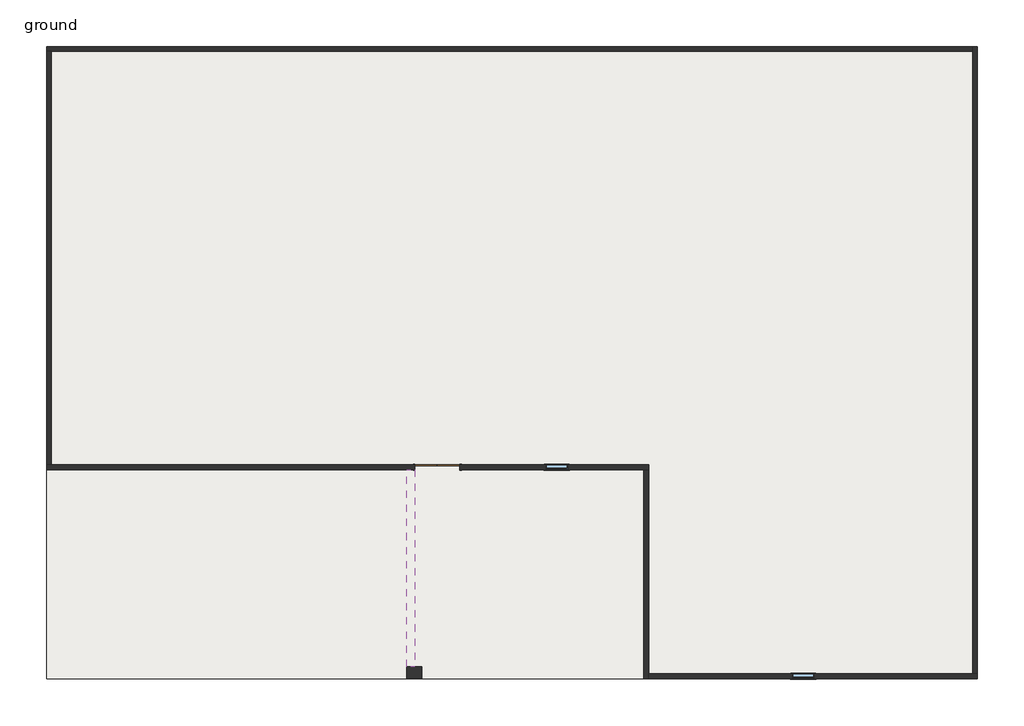
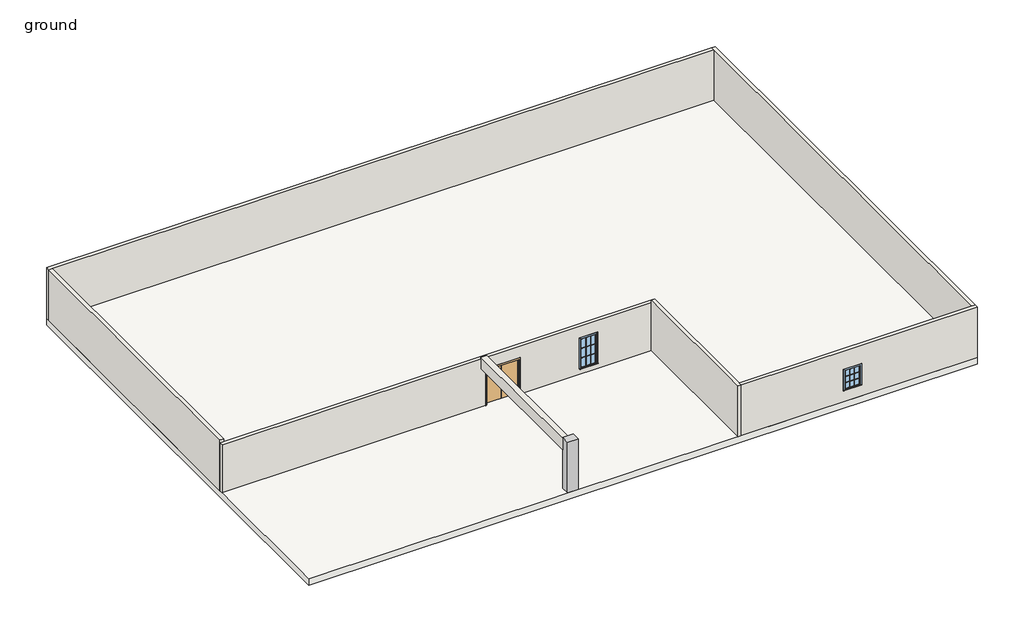
# One storey: 7 walls, 2 windows, 1 column, 1 door, 1 slab.
"""IFC4 building model written with IfcOpenShell, lengths in millimetres."""

from ifc_helpers import new_model, si_unit, frame, origin, place, context, project, spatial, polyline, outline, extrude, faceted_brep, transform, mapped, element, save
from components import m_rectangular_column_475_x_610mm_5ff218ee, door_db0c0681, walls_2_walls_2_334e7359, window_ddc5d35f, window_0c844ac8

model = new_model("IFC4")

# Units and contexts
model_context = context("Model", 3, world=origin())
ifc_project = project(units=[si_unit("LENGTHUNIT", "METRE", prefix="MILLI")], contexts=[model_context])

# Site, building, storey
site = spatial("IfcSite", under=ifc_project)
building = spatial("IfcBuilding", under=site)
storey = spatial("IfcBuildingStorey", under=building, Name="ground", Elevation=0.0)

# Column
placement = place(None, origin())
m_rectangular_column_475_x_610mm_shape = m_rectangular_column_475_x_610mm_5ff218ee(model_context)
element("IfcColumn", 1, ObjectType="M_Rectangular Column : 475 x 610mm", at=placement, inside=storey, context=model_context, shape_type="MappedRepresentation", body=[
    mapped(m_rectangular_column_475_x_610mm_shape, transform((-2824.5479903, -9080.6874979, 0.0), x_axis=(1.0, 0.0, 0.0), y_axis=(0.0, 1.0, 0.0), z_axis=(0.0, 0.0, 1.0))),
])

# Door
door_shape = door_db0c0681(model_context)
element("IfcDoor", 2, ObjectType="Door-Double-Flush_Panel : 72\" x 84\"", at=placement, inside=storey, context=model_context, shape_type="MappedRepresentation", body=[
    mapped(door_shape, transform((-1883.9625081, -698.6874979, 0.0), x_axis=(1.0, 0.0, 0.0), y_axis=(0.0, 1.0, 0.0), z_axis=(0.0, 0.0, 1.0))),
])

# Slab
element("IfcSlab", 3, ObjectType="Generic Floor - 400mm", at=placement, inside=storey, context=model_context, shape_type="SweptSolid", body=[
    extrude(outline(polyline([(20161.6374919, 16470.1125021), (20161.6374919, -9333.0874979), (-17833.5625081, -9333.0874979), (-17833.5625081, 16470.1125021), (20161.6374919, 16470.1125021)])), frame((0.0, 0.0, -400.0), z_axis=(0.0, 0.0, 1.0), x_axis=(1.0, 0.0, 0.0)), (0.0, 0.0, 1.0), 400.0),
])

# Walls
element("IfcWall", 4, ObjectType="Generic - 9\"", at=placement, inside=storey, context=model_context, shape_type="Brep", body=[
    faceted_brep([(-17833.5625081, 16270.1125021, 0.0), (-17633.5625081, 16270.1125021, 0.0), (19961.6374919, 16270.1125021, 0.0), (19961.6374919, 16270.1125021, 3048.0), (-17633.5625081, 16270.1125021, 3048.0), (-17833.5625081, 16270.1125021, 3048.0), (-17833.5625081, 16470.1125021, 0.0), (-17833.5625081, 16470.1125021, 3048.0), (19961.6374919, 16470.1125021, 3048.0), (19961.6374919, 16470.1125021, 0.0)], [[[0, 1, 2, 3, 4, 5]], [[6, 7, 8, 9]], [[2, 1, 0, 6, 9]], [[5, 4, 3, 8, 7]], [[0, 5, 7, 6]], [[3, 2, 9, 8]]]),
])
element("IfcWall", 5, ObjectType="Generic - 9\"", at=placement, inside=storey, context=model_context, shape_type="Brep", body=[
    faceted_brep([(-17633.5625081, -598.6874979, 0.0), (-17633.5625081, 16270.1125021, 0.0), (-17633.5625081, 16270.1125021, 3048.0), (-17633.5625081, -598.6874979, 3048.0), (-17833.5625081, -598.6874979, 0.0), (-17833.5625081, -598.6874979, 2870.6717354), (-17833.5625081, -598.6874979, 3048.0), (-17833.5625081, 16270.1125021, 3048.0), (-17833.5625081, 16270.1125021, 0.0)], [[[0, 1, 2, 3]], [[4, 5, 6, 7, 8]], [[1, 0, 4, 8]], [[3, 2, 7, 6]], [[2, 1, 8, 7]], [[0, 3, 6, 5, 4]]]),
])
element("IfcWall", 6, ObjectType="Generic - 9\"", at=placement, inside=storey, context=model_context, shape_type="Brep", body=[
    faceted_brep([(20161.6374919, -9133.0874979, 0.0), (19961.6374919, -9133.0874979, 0.0), (6750.4374919, -9133.0874979, 0.0), (6750.4374919, -9133.0874979, 3048.0), (19961.6374919, -9133.0874979, 3048.0), (20161.6374919, -9133.0874979, 3048.0), (12594.0374919, -9133.0874979, 1889.5975063), (12594.0374919, -9133.0874979, 670.3975063), (13508.4374919, -9133.0874979, 670.3975063), (13508.4374919, -9133.0874979, 1889.5975063), (20161.6374919, -9333.0874979, 0.0), (20161.6374919, -9333.0874979, 3048.0), (6750.4374919, -9333.0874979, 3048.0), (6750.4374919, -9333.0874979, 0.0), (12594.0374919, -9333.0874979, 1889.5975063), (13508.4374919, -9333.0874979, 1889.5975063), (13508.4374919, -9333.0874979, 670.3975063), (12594.0374919, -9333.0874979, 670.3975063)], [[[0, 1, 2, 3, 4, 5], [6, 7, 8, 9]], [[10, 11, 12, 13], [14, 15, 16, 17]], [[2, 1, 0, 10, 13]], [[5, 4, 3, 12, 11]], [[0, 5, 11, 10]], [[3, 2, 13, 12]], [[7, 6, 14, 17]], [[8, 7, 17, 16]], [[9, 8, 16, 15]], [[6, 9, 15, 14]]]),
])
element("IfcWall", 7, ObjectType="Generic - 9\"", at=placement, inside=storey, context=model_context, shape_type="Brep", body=[
    faceted_brep([(19961.6374919, 16470.1125021, 0.0), (19961.6374919, 16270.1125021, 0.0), (19961.6374919, -9133.0874979, 0.0), (19961.6374919, -9133.0874979, 3048.0), (19961.6374919, 16270.1125021, 3048.0), (19961.6374919, 16470.1125021, 3048.0), (20161.6374919, 16470.1125021, 0.0), (20161.6374919, 16470.1125021, 3048.0), (20161.6374919, -9133.0874979, 3048.0), (20161.6374919, -9133.0874979, 0.0)], [[[0, 1, 2, 3, 4, 5]], [[6, 7, 8, 9]], [[2, 1, 0, 6, 9]], [[5, 4, 3, 8, 7]], [[0, 5, 7, 6]], [[3, 2, 9, 8]]]),
])
element("IfcWall", 8, ObjectType="Generic - 9\"", at=placement, inside=storey, context=model_context, shape_type="Brep", body=[
    faceted_brep([(6750.4374919, -9333.0874979, 0.0), (6750.4374919, -9133.0874979, 0.0), (6750.4374919, -798.6874979, 0.0), (6750.4374919, -798.6874979, 2870.6717354), (6750.4374919, -798.6874979, 3048.0), (6750.4374919, -9133.0874979, 3048.0), (6750.4374919, -9333.0874979, 3048.0), (6550.4374919, -9333.0874979, 0.0), (6550.4374919, -9333.0874979, 3048.0), (6550.4374919, -798.6874979, 3048.0), (6550.4374919, -798.6874979, 0.0)], [[[0, 1, 2, 3, 4, 5, 6]], [[7, 8, 9, 10]], [[2, 1, 0, 7, 10]], [[6, 5, 4, 9, 8]], [[0, 6, 8, 7]], [[4, 3, 2, 10, 9]]]),
])
element("IfcWall", 9, ObjectType="Generic - 9\"", at=placement, inside=storey, context=model_context, shape_type="Brep", body=[
    faceted_brep([(-17833.5625081, -598.6874979, 2870.6717354), (6750.4374919, -598.6874979, 2870.6717354), (6750.4374919, -598.6874979, 0.0), (-969.5625081, -598.6874979, 0.0), (-969.5625081, -598.6874979, 2133.6), (-2798.3625081, -598.6874979, 2133.6), (-2798.3625081, -598.6874979, 0.0), (-17633.5625081, -598.6874979, 0.0), (-17833.5625081, -598.6874979, 0.0), (2535.6374919, -598.6874979, 2133.6), (2535.6374919, -598.6874979, 304.8), (3450.0374919, -598.6874979, 304.8), (3450.0374919, -598.6874979, 2133.6), (6750.4374919, -798.6874979, 2870.6717354), (-17833.5625081, -798.6874979, 2870.6717354), (-17833.5625081, -798.6874979, 0.0), (-2798.3625081, -798.6874979, 0.0), (-2798.3625081, -798.6874979, 2133.6), (-969.5625081, -798.6874979, 2133.6), (-969.5625081, -798.6874979, 0.0), (6550.4374919, -798.6874979, 0.0), (6750.4374919, -798.6874979, 0.0), (2535.6374919, -798.6874979, 2133.6), (3450.0374919, -798.6874979, 2133.6), (3450.0374919, -798.6874979, 304.8), (2535.6374919, -798.6874979, 304.8)], [[[0, 1, 2, 3, 4, 5, 6, 7, 8], [9, 10, 11, 12]], [[13, 14, 15, 16, 17, 18, 19, 20, 21], [22, 23, 24, 25]], [[15, 8, 7, 6, 16]], [[2, 21, 20, 19, 3]], [[1, 0, 14, 13]], [[0, 8, 15, 14]], [[2, 1, 13, 21]], [[18, 4, 3, 19]], [[4, 18, 17, 5]], [[5, 17, 16, 6]], [[10, 9, 22, 25]], [[11, 10, 25, 24]], [[12, 11, 24, 23]], [[9, 12, 23, 22]]]),
])
walls_2_walls_2_shape = walls_2_walls_2_334e7359(model_context)
element("IfcWall", 10, ObjectType="Walls 2 : Walls 2", at=placement, inside=storey, context=model_context, shape_type="MappedRepresentation", body=[
    mapped(walls_2_walls_2_shape, transform((0.0, 0.0, 0.0), x_axis=(1.0, 0.0, 0.0), y_axis=(0.0, 1.0, 0.0), z_axis=(0.0, 0.0, 1.0))),
])

# Windows
window_shape = window_ddc5d35f(model_context)
element("IfcWindow", 11, ObjectType="Casement 3x3 with Trim : 36\" x 48\"", at=placement, inside=storey, context=model_context, shape_type="MappedRepresentation", body=[
    mapped(window_shape, transform((13051.2374919, -9233.0874979, -244.0024937), x_axis=(-1.0, 0.0, 0.0), y_axis=(0.0, -1.0, 0.0), z_axis=(0.0, 0.0, 1.0))),
])
window_2_shape = window_0c844ac8(model_context)
element("IfcWindow", 12, ObjectType="Casement 3x3 with Trim : 36\" x 72\"", at=placement, inside=storey, context=model_context, shape_type="MappedRepresentation", body=[
    mapped(window_2_shape, transform((2992.8374919, -698.6874979, 0.0), x_axis=(-1.0, 0.0, 0.0), y_axis=(0.0, -1.0, 0.0), z_axis=(0.0, 0.0, 1.0))),
])

save(model, "model.ifc")

# Revit data of these elements
# Type "M_Rectangular Column : 475 x 610mm"
#   Depth = 1' - 6.70079"
#   Offset Base = 0' - 0"
#   Offset Top = 0' - 0"
#   Width = 2' - 0.01575"
#   Material = none
# Type "Door-Double-Flush_Panel : 72\" x 84\""
#   Type Mark = "22"
#   Construction Type Id = "DOOR"
#   Assembly Code = "C1020"
#   Analytic Construction = "Wooden"
#   Thickness = 0' - 2"
#   Thermal Resistance (R) = 0.455703 (m²·K)/W
#   Swing Angle [instance default] = 90.00°
#   Panel Width = 3' - 0"
#   Heat Transfer Coefficient (U) = 2.19465 W/(m²·K)
#   Height = 7' - 0"
#   Trim Projection Ext = 0' - 1"
#   Trim Projection Int = 0' - 1"
#   Trim Width = 0' - 3"
#   Width = 6' - 0"
#   Define Thermal Properties by = 1
#   Panel Material = Wood - Birch - Solid Stained Light Low Gloss
#   Trim Material = Paint - Sienna
#   Visual Light Transmittance = 0
#   Solar Heat Gain Coefficient = 0
#   Function = (empty or 0)
#   Wall Closure = (empty or 0)
# Type "Generic Floor - 400mm"
#   Function = 0
#   Layers, outside or top first: 1' - 3.74803" no material (function 1)
# Type "Generic - 9\""
#   Layers, outside or top first: 0' - 7.87402" no material (function 1)
# Type "Casement 3x3 with Trim : 36\" x 48\""
#   Type Mark = "19"
#   Construction Type Id = "GSP4R"
#   Assembly Code = "B2020100"
#   Analytic Construction = "1/8 in Pilkington single glazing"
#   Visual Light Transmittance = 0.9
#   Solar Heat Gain Coefficient = 0.78
#   Heat Transfer Coefficient (U) = 3.6886 W/(m²·K)
#   Height = 4' - 0"
#   Default Sill Height = 3' - 0"
#   Trim Projection - Ext. = 0' - 0 1/2"
#   Trim Projection - Int. = 0' - 0 3/4"
#   Trim Width - Exterior = 0' - 3 1/2"
#   Trim Width - Interior = 0' - 3 1/2"
#   Width = 3' - 0"
#   Window Inset = 0' - 0 3/4"
#   Define Thermal Properties by = 1
#   Glass Pane Material = Glass
#   Sash Material = Sash
#   Trim Exterior Material = Trim
#   Trim Interior Material = Trim
#   Wall Closure = (empty or 0)
# Type "Casement 3x3 with Trim : 36\" x 72\""
#   Type Mark = "21"
#   Construction Type Id = "GSP4R"
#   Assembly Code = "B2020100"
#   Analytic Construction = "1/8 in Pilkington single glazing"
#   Visual Light Transmittance = 0.9
#   Solar Heat Gain Coefficient = 0.78
#   Heat Transfer Coefficient (U) = 3.6886 W/(m²·K)
#   Height = 6' - 0"
#   Default Sill Height = 1' - 0"
#   Trim Projection - Ext. = 0' - 0 1/2"
#   Trim Projection - Int. = 0' - 0 3/4"
#   Trim Width - Exterior = 0' - 3 1/2"
#   Trim Width - Interior = 0' - 3 1/2"
#   Width = 3' - 0"
#   Window Inset = 0' - 0 3/4"
#   Define Thermal Properties by = 1
#   Glass Pane Material = Glass
#   Sash Material = Sash
#   Trim Exterior Material = Trim
#   Trim Interior Material = Trim
#   Wall Closure = (empty or 0)
# Element 1 (IfcColumn, "M_Rectangular Column : 475 x 610mm")
#   Phase Created = New Construction
# Element 2 (IfcDoor, "Door-Double-Flush_Panel : 72\" x 84\"")
#   Swing Angle = 90.00°
#   Phase Created = New Construction
#   Materials on its faces: "Paint - Sienna", "Wood - Birch - Solid Stained Light Low Gloss"
# Element 3 (IfcSlab, "Generic Floor - 400mm")
#   Height Offset From Level = 0' - 0"
#   Phase Created = New Construction
#   Materials on its faces: "Default Roof"
# Elements 4, 5, 6, 7, 8 (IfcWall, "Generic - 9\"")
#   Top Offset = 0' - 0"
#   Base Offset = 0' - 0"
#   Unconnected Height = 10' - 0"
#   wall height = 10' - 0"
#   Phase Created = New Construction
#   Base Constraint = ground
#   Materials on its faces: "Default Wall"
# Element 9 (IfcWall, "Generic - 9\"")
#   Top Offset = 0' - 0"
#   Base Offset = 0' - 0"
#   Unconnected Height = 9' - 5.01857"
#   wall height = 9' - 5.01857"
#   Phase Created = New Construction
#   Base Constraint = ground
#   Materials on its faces: "Default Wall"
# Element 10 (IfcWall, "Walls 2 : Walls 2")
#   Phase Created = New Construction
#   Materials on its faces: "Default Wall"
# Element 11 (IfcWindow, "Casement 3x3 with Trim : 36\" x 48\"")
#   Mark = "9"
#   Phase Created = New Construction
#   Materials on its faces: "Sash", "Glass", "Trim"
# Element 12 (IfcWindow, "Casement 3x3 with Trim : 36\" x 72\"")
#   Mark = "6"
#   Phase Created = New Construction
#   Materials on its faces: "Sash", "Glass", "Trim"
# Materials
#   "Wood - Birch - Solid Stained Light Low Gloss": class "Wood", colour RGB 210 159 95, transparency 0, Cost = 0
#   "Paint - Sienna": colour RGB 118 70 51, transparency 0, Cost = 0
#   "Glass": class "Glass", colour RGB 218 227 224, transparency 0.85, Description = "Soda Lime Glass", Cost = 0
#   "Sash": class "Wood", colour RGB 136 99 55, transparency 0
#   "Trim": class "Wood", colour RGB 224 178 126, transparency 0
#   "Default Roof": colour RGB 80 80 80, transparency 0
#   "Default Wall": colour RGB 80 80 80, transparency 0
